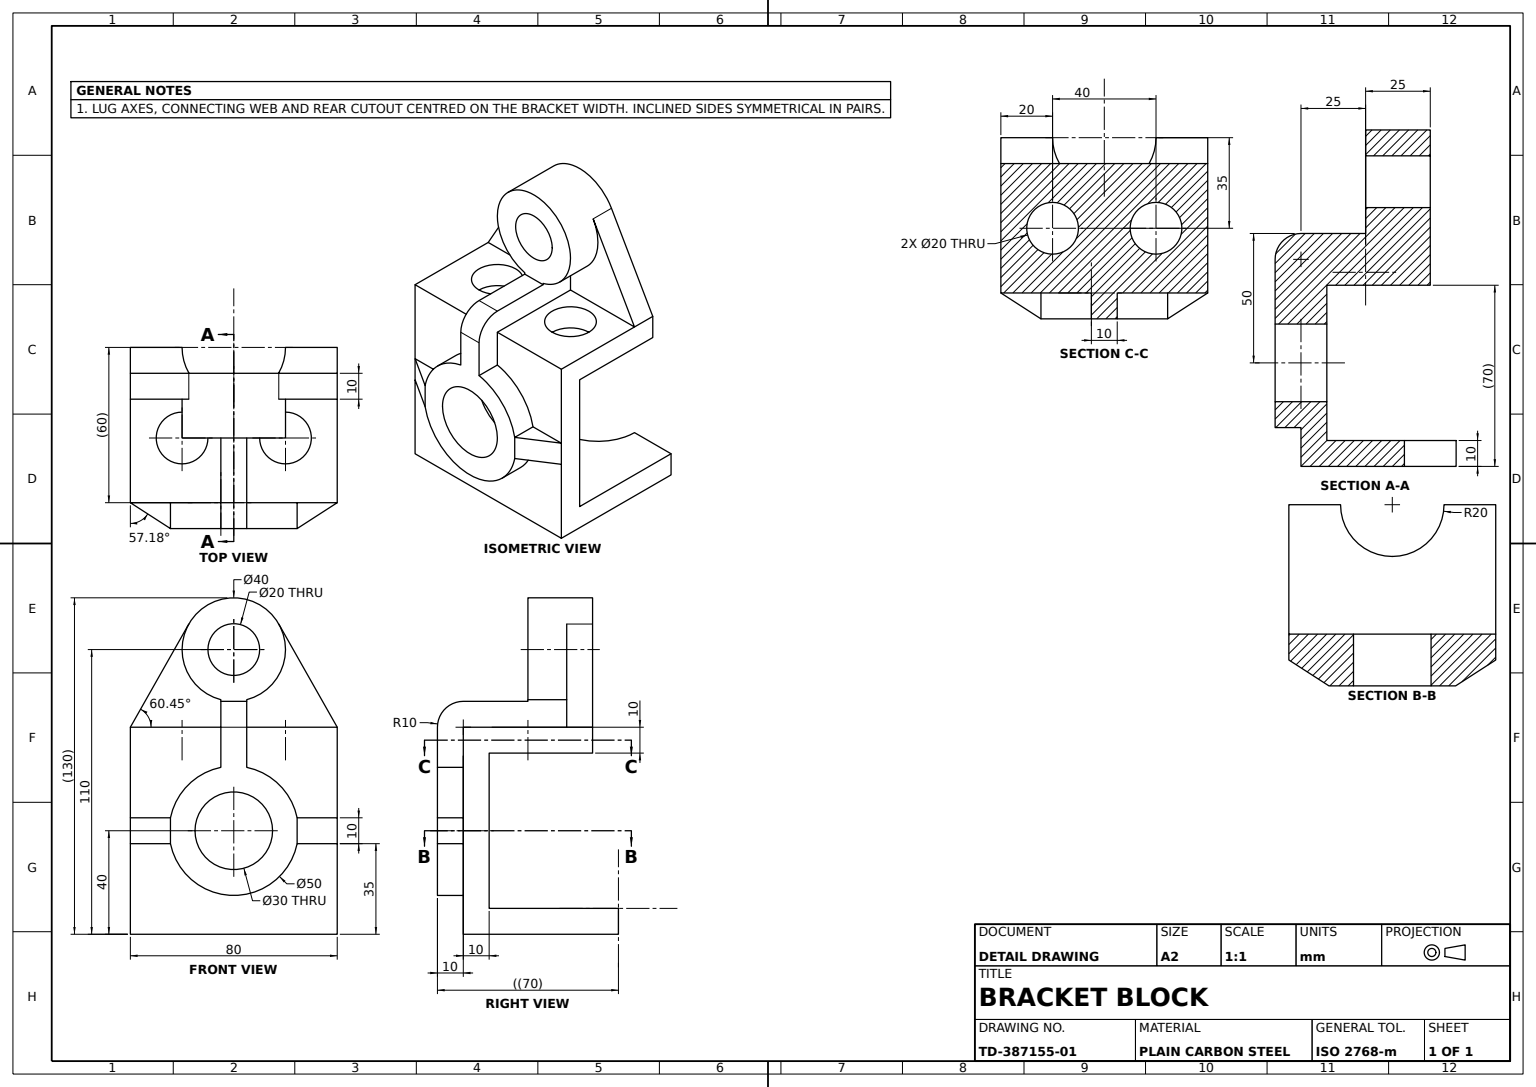
from build123d import *

# Parameters (mm, degrees)
BASE_BRACKET_80MM_DEPTH   = 40
UPPER_LUG_PLATE_DEPTH     = 10
SKETCH2_3_R               = 20
SKETCH2_3_R_2             = 10
UPPER_LUG_HUB_DEPTH       = 25
FRONT_LUG_PROFILE_R       = 25
FRONT_LUG_PROFILE_R_2     = 15
FRONT_LUG_BOSS_DEPTH      = 10
FRONT_LUG_BORE_REACH      = 150.661
SKETCH4_2_R               = 15
CONNECTING_WEB_DEPTH      = 5
WEB_PAD_A_PROFILE_W       = 10
WEB_PAD_A_PROFILE_H       = 10
WEB_PAD_A_DEPTH           = 5
WEB_PAD_B_PROFILE_W       = 10
WEB_PAD_B_PROFILE_H       = 50
WEB_PAD_B_DEPTH           = 5
WEB_RELIEF_CUT_REACH      = 152.083
WEB_RELIEF_PROFILE_W      = 35
WEB_RELIEF_PROFILE_H      = 5
WEB_RELIEF_FILLET_R10_R   = 10
GUSSET_RIB_DEPTH          = 5
RIB_TRIM_CUT_REACH        = 113.467
RIB_PAD_A_DEPTH           = 5
RIB_PAD_B_DEPTH           = 5
LUG_CLEARANCE_CUT_REACH   = 154.971
RIB_NOTCH_CUT_DEPTH       = 10
UPPER_HUB_BORE_20_REACH   = 109.703
UPPER_HUB_BORE_PROFILE_R  = 10
BASE_ARC_CUTOUT_REACH     = 142
BASE_ARC_CUTOUT_PROFILE_R = 20


with BuildPart() as part:
    # Base Bracket Profile → Base Bracket 80mm (new, symmetric)
    with BuildSketch(Plane(origin=(0, 0, 0), x_dir=(0, 0, -1), z_dir=(1, 0, 0))):
        Polygon((0, 0), (60, 0), (60, 10), (10, 10), (10, 70), (50, 70), (50, 80), (0, 80), align=None)
    extrude(amount=BASE_BRACKET_80MM_DEPTH, both=True)

    # Upper Lug Profile → Upper Lug Plate (add)
    with BuildSketch(Plane(origin=(0, 0, -50), x_dir=(-1, 0, 0), z_dir=(0, 0, -1))):
        with BuildLine():
            Line((-40, 80), (0, 80))
            Line((0, 80), (0, 90))
            ThreePointArc((0, 90), (-17.281273745, 99.932349938), (-17.398181668, 119.864242224))
            Line((-17.398181668, 119.864242224), (-40, 80))
        make_face()
        with BuildLine():
            Line((0, 90), (0, 80))
            Line((0, 80), (40, 80))
            Line((40, 80), (17.398181668, 119.864242224))
            ThreePointArc((17.398181668, 119.864242224), (19.338609482, 115.100802223), (20, 110))
            ThreePointArc((20, 110), (14.142135624, 95.857864376), (0, 90))
        make_face()
    extrude(amount=-UPPER_LUG_PLATE_DEPTH)

    # Sketch2_3 → Upper Lug Hub (add)
    with BuildSketch(Plane(origin=(0, 0, -50), x_dir=(-1, 0, 0), z_dir=(0, 0, -1))):
        with Locations((0, 110)):
            Circle(SKETCH2_3_R)
        with Locations((0, 110)):
            Circle(SKETCH2_3_R_2, mode=Mode.SUBTRACT)
    extrude(amount=-UPPER_LUG_HUB_DEPTH)

    # Front Lug Profile → Front Lug Boss (add)
    with BuildSketch(Plane.XY):
        with Locations((0, 40)):
            Circle(FRONT_LUG_PROFILE_R)
        with Locations((0, 40)):
            Circle(FRONT_LUG_PROFILE_R_2, mode=Mode.SUBTRACT)
    extrude(amount=FRONT_LUG_BOSS_DEPTH)

    # Sketch4_2 → Front Lug Bore (cut, up to next)
    with BuildSketch(Plane.XY, mode=Mode.PRIVATE) as front_lug_bore_sk1:
        with Locations((0, 40)):
            Circle(SKETCH4_2_R)
    front_lug_bore_tool1 = extrude(front_lug_bore_sk1.sketch, amount=-FRONT_LUG_BORE_REACH, mode=Mode.PRIVATE) & part.part
    add(front_lug_bore_tool1.solids().sort_by_distance((0, 40, 0))[0], mode=Mode.SUBTRACT)



with BuildPart() as body_2:
    # Connecting Web Profile → Connecting Web (new, symmetric)
    with BuildSketch(Plane(origin=(0, 0, 0), x_dir=(0, 0, -1), z_dir=(1, 0, 0))):
        Polygon((-10, 66.461599877), (-10, 90), (40, 90), (40, 80), (0, 80), (0, 66.461599877), align=None)
    extrude(amount=CONNECTING_WEB_DEPTH, both=True)


with BuildPart() as body_3:
    # Web Pad A Profile → Web Pad A (new, symmetric)
    with BuildSketch(Plane.XZ.offset(-66.461599877)):
        with Locations((0, 5)):
            Rectangle(WEB_PAD_A_PROFILE_W, WEB_PAD_A_PROFILE_H)
    extrude(amount=WEB_PAD_A_DEPTH, both=True)


with BuildPart() as part_1:
    add(part.part)

    add(body_2.part)  # Web Pad B merges body 2
    # Web Pad B Profile → Web Pad B (add, symmetric)
    with BuildSketch(Plane(origin=(0, 90, 0), x_dir=(1, 0, 0), z_dir=(0, 1, 0))):
        with Locations((0, 15)):
            Rectangle(WEB_PAD_B_PROFILE_W, WEB_PAD_B_PROFILE_H)
    extrude(amount=WEB_PAD_B_DEPTH, both=True)

    # Combine Web Pads: union body 3
    add(body_3.part)

    # Web Relief Profile → Web Relief Cut (cut, up to next)
    with BuildSketch(Plane(origin=(5, 0, 0), x_dir=(0, 0, -1), z_dir=(1, 0, 0)), mode=Mode.PRIVATE) as web_relief_cut_sk1:
        with Locations((7.5, 92.5)):
            Rectangle(WEB_RELIEF_PROFILE_W, WEB_RELIEF_PROFILE_H)
    web_relief_cut_tool1 = extrude(web_relief_cut_sk1.sketch, amount=-WEB_RELIEF_CUT_REACH, mode=Mode.PRIVATE) & part_1.part
    add(web_relief_cut_tool1.solids().sort_by_distance((5, 92.5, -7.5))[0], mode=Mode.SUBTRACT)

    # Web Relief Fillet R10
    web_relief_fillet_r10_edges = [part_1.edges().sort_by_distance(p)[0] for p in [
        (0, 90, 10),
    ]]
    fillet(web_relief_fillet_r10_edges, radius=WEB_RELIEF_FILLET_R10_R)

    # Gusset Rib Path → Gusset Rib (add, symmetric)
    with BuildSketch(Plane(origin=(0, 40, 0), x_dir=(-1, 0, 0), z_dir=(0, -1, 0))):
        Polygon((-25, -10), (-40, 0), (-34.452998038, 8.320502943), (-19.452998038, -1.679497057), align=None)
    gusset_rib = extrude(amount=GUSSET_RIB_DEPTH, both=True)

    # Rib Trim Profile → Rib Trim Cut (cut, up to next)
    with BuildSketch(Plane(origin=(0, 45, 0), x_dir=(1, 0, 0), z_dir=(0, 1, 0)), mode=Mode.PRIVATE) as rib_trim_cut_sk1:
        Polygon((24.494897428, -10), (40, 0), (25, -10), align=None)
    rib_trim_cut_tool1 = extrude(rib_trim_cut_sk1.sketch, amount=-RIB_TRIM_CUT_REACH, mode=Mode.PRIVATE) & part_1.part
    rib_trim_cut = rib_trim_cut_tool1.solids().sort_by_distance((29.831632, 45, 6.666667))[0]
    add(rib_trim_cut, mode=Mode.SUBTRACT)

    # Rib Pad A Profile → Rib Pad A (add, symmetric)
    with BuildSketch(Plane(origin=(12.692307692, 0, -8.461538462), x_dir=(0.5547001962252294, 0, 0.8320502943378436), z_dir=(-0.8320502943378436, 0, 0.5547001962252294))):
        with BuildLine():
            Line((21.277421237, 35), (21.91421024, 35))
            Line((21.91421024, 35), (21.91421024, 37.248507099))
            add(Edge.make_bspline(
                [(21.277421237, 35), (21.688173728, 36.116205467), (21.91421024, 37.248507099)],
                knots=[2.940234733, 2.940234733, 2.940234733, 3.031309523, 3.031309523, 3.031309523], degree=2, weights=[1, 0.998963352, 1]))
        make_face()
    rib_pad_a = extrude(amount=RIB_PAD_A_DEPTH, both=True)

    # Rib Pad B Profile → Rib Pad B (add, symmetric)
    with BuildSketch(Plane(origin=(12.692307692, 0, -8.461538462), x_dir=(0.5547001962252294, 0, 0.8320502943378436), z_dir=(-0.8320502943378436, 0, 0.5547001962252294))):
        with BuildLine():
            Line((21.91421024, 42.751492901), (21.91421024, 45))
            Line((21.91421024, 45), (21.277421237, 45))
            add(Edge.make_bspline(
                [(21.91421024, 42.751492901), (21.688173728, 43.883794533), (21.277421237, 45)],
                knots=[3.251875784, 3.251875784, 3.251875784, 3.342950574, 3.342950574, 3.342950574], degree=2, weights=[1, 0.998963352, 1]))
        make_face()
    rib_pad_b = extrude(amount=RIB_PAD_B_DEPTH, both=True)

    # Lug Clearance Cut: up to this plane
    lug_clearance_cut_end = Plane(origin=(20.687872941, 35, 12.5456876), z_dir=(-0.5547001962252294, 0, -0.8320502943378436))
    # Lug Clearance Profile → Lug Clearance Cut (cut, up to the surface)
    with BuildSketch(Plane.XY.offset(10), mode=Mode.PRIVATE) as lug_clearance_cut_sk1:
        with BuildLine():
            Line((24.494897428, 37.216718732), (24.494897428, 35))
            ThreePointArc((24.494897428, 35), (-17.67766953, 22.32233047), (-5, 64.494897428))
            Line((-5, 64.494897428), (-5, 80))
            Line((-5, 80), (5, 80))
            Line((5, 80), (5, 64.494897428))
            ThreePointArc((5, 64.494897428), (17.67766953, 57.67766953), (24.494897428, 45))
            Line((24.494897428, 45), (24.494897428, 37.216718732))
        make_face()
    lug_clearance_cut_tool1 = split(extrude(lug_clearance_cut_sk1.sketch, amount=LUG_CLEARANCE_CUT_REACH, mode=Mode.PRIVATE), bisect_by=lug_clearance_cut_end, keep=Keep.BOTH, mode=Mode.PRIVATE)
    lug_clearance_cut = lug_clearance_cut_tool1.solids().sort_by_distance((-0.039461, 42.32819, 10))[0]
    add(lug_clearance_cut, mode=Mode.SUBTRACT)

    # Rib Notch Profile → Rib Notch Cut (cut)
    with BuildSketch(Plane.XZ.offset(-35)):
        Polygon((24.848124412, 9.772186619), (24.494897428, 10), (24.494897428, 10.007671275), align=None)
    rib_notch_cut = extrude(amount=-RIB_NOTCH_CUT_DEPTH, mode=Mode.SUBTRACT)

    # Rib Features Mirror: Gusset Rib, Rib Trim Cut, Rib Pad A, Rib Pad B, Lug Clearance Cut, Rib Notch Cut across plane
    add(gusset_rib.mirror(Plane(origin=(0, 0, 0), x_dir=(0, 0, 1), z_dir=(1, 0, 0))))
    add(rib_trim_cut.mirror(Plane(origin=(0, 0, 0), x_dir=(0, 0, 1), z_dir=(1, 0, 0))), mode=Mode.SUBTRACT)
    add(rib_pad_a.mirror(Plane(origin=(0, 0, 0), x_dir=(0, 0, 1), z_dir=(1, 0, 0))))
    add(rib_pad_b.mirror(Plane(origin=(0, 0, 0), x_dir=(0, 0, 1), z_dir=(1, 0, 0))))
    add(lug_clearance_cut.mirror(Plane(origin=(0, 0, 0), x_dir=(0, 0, 1), z_dir=(1, 0, 0))), mode=Mode.SUBTRACT)
    add(rib_notch_cut.mirror(Plane(origin=(0, 0, 0), x_dir=(0, 0, 1), z_dir=(1, 0, 0))), mode=Mode.SUBTRACT)

    # Upper Hub Bore Profile → Upper Hub Bore _20 (cut, up to next)
    with BuildSketch(Plane(origin=(0, 80, 0), x_dir=(1, 0, 0), z_dir=(0, 1, 0)), mode=Mode.PRIVATE) as upper_hub_bore_20_sk1:
        with Locations(Location((-20, 25, 0), (0, 0, 270))):
            Circle(UPPER_HUB_BORE_PROFILE_R)
    upper_hub_bore_20_tool1 = extrude(upper_hub_bore_20_sk1.sketch, amount=-UPPER_HUB_BORE_20_REACH, mode=Mode.PRIVATE) & part_1.part
    # Upper Hub Bore Profile → Upper Hub Bore _20 (cut, up to next)
    with BuildSketch(Plane(origin=(0, 80, 0), x_dir=(1, 0, 0), z_dir=(0, 1, 0)), mode=Mode.PRIVATE) as upper_hub_bore_20_sk2:
        with Locations(Location((20, 25, 0), (0, 0, 270))):
            Circle(UPPER_HUB_BORE_PROFILE_R)
    upper_hub_bore_20_tool2 = extrude(upper_hub_bore_20_sk2.sketch, amount=-UPPER_HUB_BORE_20_REACH, mode=Mode.PRIVATE) & part_1.part
    add(upper_hub_bore_20_tool1.solids().sort_by_distance((-20, 80, -25))[0], mode=Mode.SUBTRACT)
    add(upper_hub_bore_20_tool2.solids().sort_by_distance((20, 80, -25))[0], mode=Mode.SUBTRACT)

    # Base Arc Cutout Profile → Base Arc Cutout (cut, up to next)
    with BuildSketch(Plane(origin=(0, 10, 0), x_dir=(1, 0, 0), z_dir=(0, 1, 0)), mode=Mode.PRIVATE) as base_arc_cutout_sk1:
        with Locations((0, 60)):
            Circle(BASE_ARC_CUTOUT_PROFILE_R)
    base_arc_cutout_tool1 = extrude(base_arc_cutout_sk1.sketch, amount=-BASE_ARC_CUTOUT_REACH, mode=Mode.PRIVATE) & part_1.part
    add(base_arc_cutout_tool1.solids().sort_by_distance((0, 10, -60))[0], mode=Mode.SUBTRACT)


solid = part_1.part
